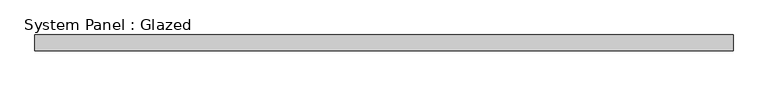
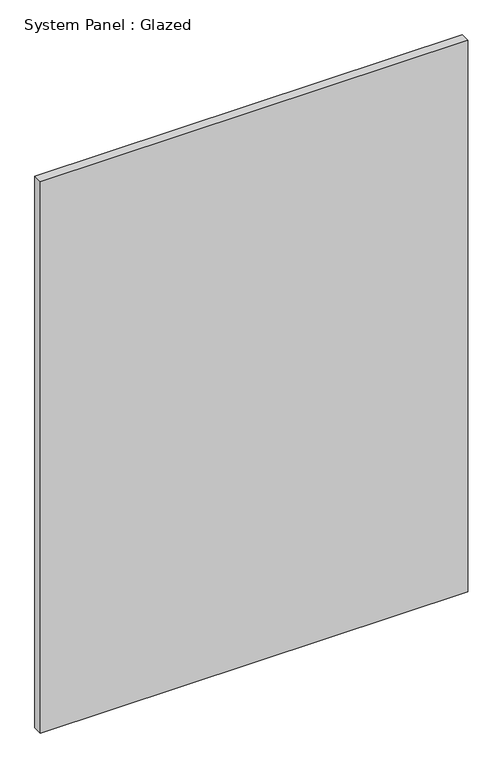
"""IFC4 building model written with IfcOpenShell, lengths in millimetres: plate geometry, System Panel : Glazed."""

from ifc_helpers import new_model, si_unit, origin, origin_with_axes, place, context, project, spatial, polyline, outline, extrude, source, transform, mapped, element, save


def system_panel_glazed_9bd642df(model_context):
    return source(origin(), model_context, "Body", "SweptSolid", [
        extrude(outline(polyline([(563.3718553, 19.05), (-563.3718553, 19.05), (-563.3718553, 44.45), (563.3718553, 44.45), (563.3718553, 19.05)])), origin_with_axes(), (0.0, 0.0, 1.0), 1535.7829369),
    ])


if __name__ == "__main__":
    model = new_model("IFC4")
    model_context = context("Model", 3, world=origin())
    ifc_project = project(units=[si_unit("LENGTHUNIT", "METRE", prefix="MILLI")], contexts=[model_context])
    site = spatial("IfcSite", under=ifc_project)
    building = spatial("IfcBuilding", under=site)
    placement = place(None, origin())
    system_panel_glazed_shape = system_panel_glazed_9bd642df(model_context)
    element("IfcPlate", 1, ObjectType="System Panel : Glazed", at=placement, inside=building, context=model_context, shape_type="MappedRepresentation", body=[
        mapped(system_panel_glazed_shape, transform((0.0, 0.0, 0.0), x_axis=(1.0, 0.0, 0.0), y_axis=(0.0, 1.0, 0.0), z_axis=(0.0, 0.0, 1.0))),
    ])
    save(model, "model.ifc")

# Revit data of these elements
# Type "System Panel : Glazed"
#   Construction Type Id = "GSP4R"
#   Analytic Construction = "1/8 in Pilkington single glazing"
#   Visual Light Transmittance = 0.9
#   Solar Heat Gain Coefficient = 0.86
#   Heat Transfer Coefficient (U) = 1.18115 BTU/(h·ft²·°F)
#   Define Thermal Properties by = 1
# Element 1 (IfcPlate, "System Panel : Glazed")
#   Materials on its faces: "Glass"
# Materials
#   "Glass": class "Glass", colour RGB 0 128 192, transparency 0.75, Description = "Soda Lime Glass", Cost = 0
